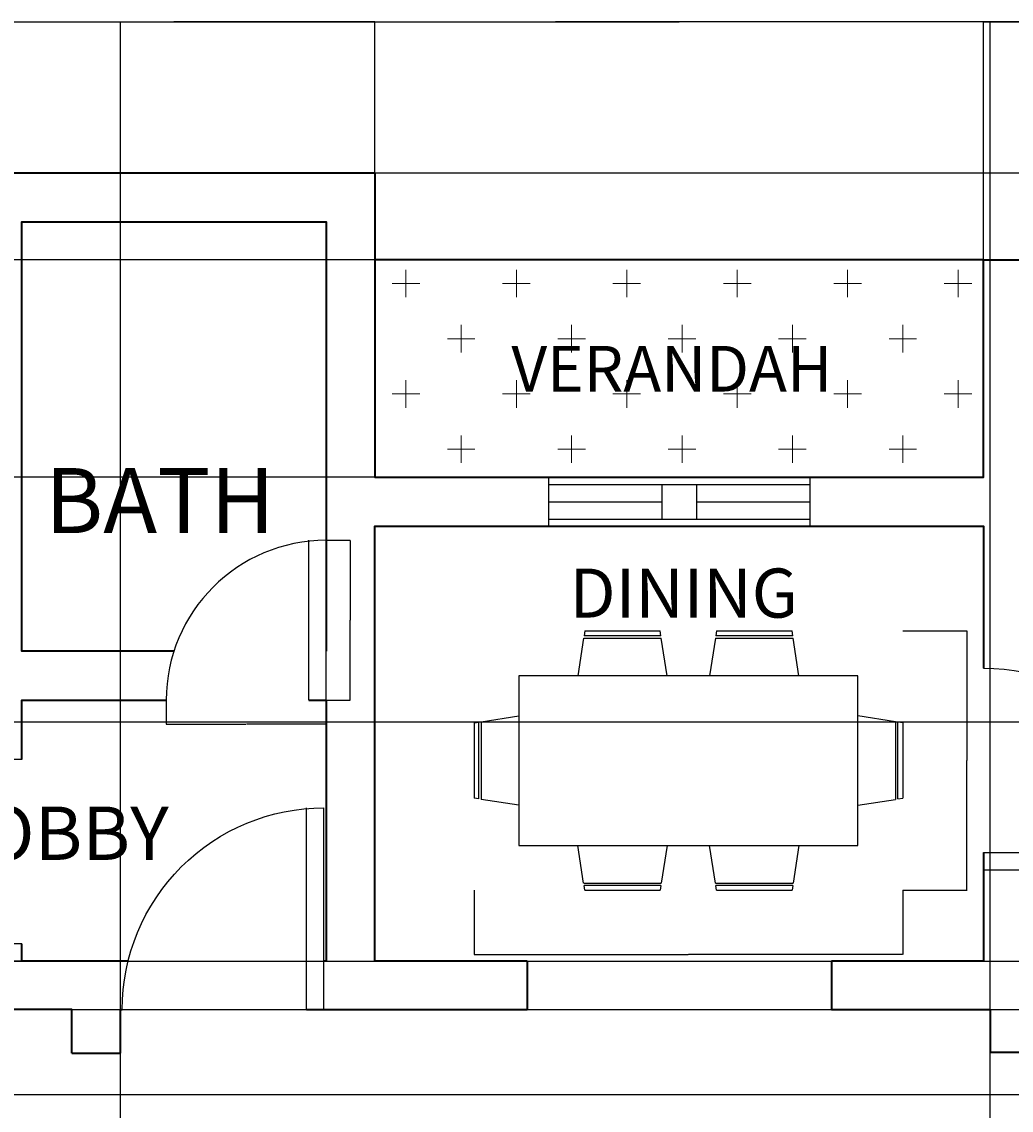
# Model space of a CAD drawing. Units: millimetres. Extents: x 19292 to 100733, y 12374 to 26974.
# Tile 17 of 24: x 26744 to 31296, y 18550 to 23556. Entities that reach past the tile are written whole.
import ezdxf

# ---------------------------------------------------------------- set-up
doc = ezdxf.new("R2010")
doc.units = ezdxf.units.MM
for name, color, linetype, lineweight in [('A-ANNO-DIMS', 2, 'Continuous', 18), ('A-AREA-IDEN', 3, 'Continuous', 25), ('A-DOOR', 4, 'Continuous', 25), ('A-FLOR-PATT', 252, 'Continuous', 13), ('A-FURN', 8, 'Continuous', 18), ('A-GLAZ', 3, 'Continuous', 25), ('A-WALL', 7, 'Continuous', 35)]:
    doc.layers.add(name, color=color, linetype=linetype, lineweight=lineweight)
doc.layers.add('FURNITURE', color=40, linetype='Continuous')
doc.layers.add('WINDOWS', color=50, linetype='Continuous')
doc.styles.get("Standard").update_dxf_attribs({"font": 'arial.ttf'})
doc.dimstyles.get("Standard").update_dxf_attribs({"dimtxt": 0.18, "dimasz": 0.18, "dimexe": 0.18, "dimexo": 0.0625, "dimgap": 0.09, "dimtad": 0, "dimtih": 1, "dimtoh": 1, "dimdec": 4, "dimzin": 0, "dimdsep": 46, "dimtxsty": 'Standard', "dimcen": 0.09, "dimadec": 0, "dimazin": 0, "dimtfac": 1, "dimtdec": 4, "dimtofl": 0, "dimtmove": 0, "dimatfit": 3, "dimfxl": 1, "dimtolj": 1, "dimtzin": 0, "dimarcsym": 0})

# ---------------------------------------------------------------- blocks, each defined once
blk = doc.blocks.new('WW')
at = {"layer": 'WINDOWS'}
for p, q in [((-5183.9, -4940.9), (-3983.9, -4940.9)), ((-4663.9, -4940.9), (-4663.9, -5100.9)), ((-4503.9, -4940.9), (-4503.9, -5100.9)), ((-4503.9, -4940.9), (-4503.9, -5100.9)), ((-5183.9, -5020.9), (-4663.9, -5020.9)), ((-4503.9, -5020.9), (-3983.9, -5020.9)), ((-5183.9, -5100.9), (-3983.9, -5100.9))]:
    blk.add_line(p, q, dxfattribs=at)
for points in [[(-5183.9, -5133.4), (-5183.9, -4908.4)], [(-3983.9, -4908.4), (-3983.9, -5133.4)]]:
    blk.add_lwpolyline(points, dxfattribs=at)
blk = doc.blocks.new('6X3DINING')
at = {"layer": 'FURNITURE'}
for p, q in [((13.7657, 44.00059), (12.5153, 35.99762)), ((13.7696, 44), (30.2392, 44)), ((14, 45.5), (13.8438, 44.50042)), ((30.1584, 44.5), (13.8466, 44.5)), ((14, 45.5), (30, 45.5)), ((30.1563, 44.49966), (30, 45.5)), ((31.4848, 35.99762), (30.2345, 43.99926)), ((41.7657, 44.00059), (40.5153, 35.99762)), ((41.7696, 44), (58.2392, 44)), ((42, 45.5), (41.8438, 44.50042)), ((58.1584, 44.5), (41.8466, 44.5)), ((42, 45.5), (58, 45.5)), ((58.1563, 44.49966), (58, 45.5)), ((59.4848, 35.99762), (58.2345, 43.99926)), ((72, 36), (0, 36)), ((0, 36), (0, 0)), ((72, 0), (72, 36)), ((-9.5, 26), (-8.5004, 26.15617)), ((-9.5, 26), (-9.5, 10)), ((-8.5, 9.84157), (-8.5, 26.15338)), ((-8.0006, 26.23428), (0.0024, 27.48474)), ((-8, 26.23041), (-8, 9.76085)), ((80.0006, 26.23428), (71.9976, 27.48474)), ((80, 26.23041), (80, 9.76085)), ((80.5, 9.84157), (80.5, 26.15338)), ((81.5, 26), (80.5005, 26.15617)), ((81.5, 26), (81.5, 10)), ((-8.4997, 9.84369), (-9.5, 10)), ((0.0024, 8.51524), (-7.9993, 9.7655)), ((71.9976, 8.51524), (79.9993, 9.7655)), ((80.4997, 9.84369), (81.5, 10)), ((0, 0), (72, 0)), ((13.7657, -8.0006), (12.5153, 0.00238)), ((31.4848, 0.00238), (30.2345, -7.99928)), ((41.7657, -8.0006), (40.5153, 0.00238)), ((59.4848, 0.00238), (58.2345, -7.99928)), ((13.7696, -8), (30.2392, -8)), ((14, -9.5), (13.8438, -8.50044)), ((30.1584, -8.5), (13.8466, -8.5)), ((30.1563, -8.49967), (30, -9.5)), ((41.7696, -8), (58.2392, -8)), ((42, -9.5), (41.8438, -8.50044)), ((58.1584, -8.5), (41.8466, -8.5)), ((58.1563, -8.49967), (58, -9.5)), ((14, -9.5), (30, -9.5)), ((42, -9.5), (58, -9.5))]:
    blk.add_line(p, q, dxfattribs=at)
blk = doc.blocks.new('DOOR-900')
for p, q in [((927.7, 80), (0, 80)), ((927.7, 0), (927.7, 80)), ((927.7, 0), (927.7, 80)), ((927.7, 0), (0, 0))]:
    blk.add_line(p, q)
blk.add_arc((927.7, 0), 927.7, 90, 180)
blk = doc.blocks.new('DOOR-750')
for p, q in [((655.3, 0), (655.3, 735.3)), ((735.3, 0), (735.3, 735.3)), ((735.3, 0), (655.3, 0)), ((735.3, 0), (655.3, 0))]:
    blk.add_line(p, q)
blk.add_arc((735.3, 0), 735.3, 90, 180)
blk = doc.blocks.new('DOOR-SWING-900')
blk.add_line((927.7, 927.7), (927.7, 0))
blk.add_arc((927.7, 927.7), 927.7, 180, 270)
blk = doc.blocks.new('*D30')
at = {"layer": 'A-ANNO-DIMS', "color": 0, "lineweight": -2, "transparency": 16777216}
for p, q in [((27408.9, 20435.7), (27408.9, 20325.3)), ((28144.1, 20435.7), (28144.1, 20325.3)), ((27409, 20325.4), (27775.2, 20325.4)), ((28144, 20325.4), (27777.7, 20325.4))]:
    blk.add_line(p, q, dxfattribs=at)
at = {"layer": 'A-ANNO-DIMS', "color": 0, "transparency": 16777216}
for points in [[(27409, 20325.5), (27409, 20325.4), (27408.9, 20325.4)], [(28144, 20325.5), (28144, 20325.4), (28144.1, 20325.4)]]:
    blk.add_solid(points, dxfattribs=at)
at = {"layer": 'Defpoints', "color": 0, "transparency": 16777216}
for p in [(27408.9, 20435.7), (28144.1, 20435.7), (28144.1, 20325.4)]:
    blk.add_point(p, dxfattribs=at)
at = {"layer": 'A-ANNO-DIMS', "color": 0, "transparency": 16777216, "insert": (27776.5, 20325.4), "char_height": 0.18, "attachment_point": 5}
blk.add_mtext('\\A1;DOOR 750 735 TYP.', dxfattribs=at)
blk = doc.blocks.new('*D31')
at = {"layer": 'A-ANNO-DIMS', "color": 0, "lineweight": -2, "transparency": 16777216}
for p, q in [((28144.2, 21171), (28254.6, 21171)), ((28254.4, 21170.8), (28254.4, 20803.5)), ((28254.4, 20435.9), (28254.4, 20803.2)), ((28144.2, 20435.7), (28254.6, 20435.7))]:
    blk.add_line(p, q, dxfattribs=at)
at = {"layer": 'A-ANNO-DIMS', "color": 0, "transparency": 16777216}
for points in [[(28254.4, 21170.8), (28254.5, 21170.8), (28254.4, 21171)], [(28254.4, 20435.9), (28254.5, 20435.9), (28254.4, 20435.7)]]:
    blk.add_solid(points, dxfattribs=at)
at = {"layer": 'Defpoints', "color": 0, "transparency": 16777216}
for p in [(28144.1, 21171), (28254.4, 21171), (28144.1, 20435.7)]:
    blk.add_point(p, dxfattribs=at)
at = {"layer": 'A-ANNO-DIMS', "color": 0, "transparency": 16777216, "insert": (28254.4, 20803.4), "char_height": 0.18, "attachment_point": 5}
blk.add_mtext('\\A1;735 TYP.', dxfattribs=at)
blk = doc.blocks.new('*D50')
at = {"layer": 'A-ANNO-DIMS', "color": 0, "lineweight": -2, "transparency": 16777216}
for p, q in [((28825.2, 19562.1), (28825.2, 19266.2)), ((30797.1, 19562.1), (30797.1, 19266.2)), ((28825.3, 19266.4), (29810, 19266.4)), ((30796.9, 19266.4), (29812.2, 19266.4))]:
    blk.add_line(p, q, dxfattribs=at)
at = {"layer": 'A-ANNO-DIMS', "color": 0, "transparency": 16777216}
for points in [[(28825.3, 19266.4), (28825.3, 19266.4), (28825.2, 19266.4)], [(30796.9, 19266.4), (30796.9, 19266.4), (30797.1, 19266.4)]]:
    blk.add_solid(points, dxfattribs=at)
at = {"layer": 'Defpoints', "color": 0, "transparency": 16777216}
for p in [(28825.2, 19562.2), (30797.1, 19562.2), (30797.1, 19266.4)]:
    blk.add_point(p, dxfattribs=at)
at = {"layer": 'A-ANNO-DIMS', "color": 0, "transparency": 16777216, "insert": (29811.1, 19266.4), "char_height": 0.18, "attachment_point": 5}
blk.add_mtext('\\A1;DINING SET 1972', dxfattribs=at)
blk = doc.blocks.new('*D51')
at = {"layer": 'A-ANNO-DIMS', "color": 0, "lineweight": -2, "transparency": 16777216}
for p, q in [((30797.1, 20754), (31093, 20754)), ((31092.8, 20753.8), (31092.8, 20158.2)), ((31092.8, 19562.3), (31092.8, 20157.9)), ((30797.1, 19562.2), (31093, 19562.2))]:
    blk.add_line(p, q, dxfattribs=at)
at = {"layer": 'A-ANNO-DIMS', "color": 0, "transparency": 16777216}
for points in [[(31092.8, 20753.8), (31092.9, 20753.8), (31092.8, 20754)], [(31092.8, 19562.3), (31092.9, 19562.3), (31092.8, 19562.2)]]:
    blk.add_solid(points, dxfattribs=at)
at = {"layer": 'Defpoints', "color": 0, "transparency": 16777216}
for p in [(30797.1, 20754), (31092.8, 20754), (30797.1, 19562.2)]:
    blk.add_point(p, dxfattribs=at)
at = {"layer": 'A-ANNO-DIMS', "color": 0, "transparency": 16777216, "insert": (31092.8, 20158.1), "char_height": 0.18, "attachment_point": 5}
blk.add_mtext('\\A1;1192', dxfattribs=at)
blk = doc.blocks.new('*D61')
at = {"layer": 'A-ANNO-DIMS', "color": 0, "lineweight": -2, "transparency": 16777216}
for p, q in [((26519.1, 22635.8), (26519.1, 23555.9)), ((26519.3, 23555.7), (27443.8, 23555.7)), ((28369, 23555.7), (27444.5, 23555.7)), ((28369.1, 22860.8), (28369.1, 23555.9))]:
    blk.add_line(p, q, dxfattribs=at)
at = {"layer": 'A-ANNO-DIMS', "color": 0, "transparency": 16777216}
for points in [[(26519.3, 23555.8), (26519.3, 23555.7), (26519.1, 23555.7)], [(28369, 23555.8), (28369, 23555.7), (28369.1, 23555.7)]]:
    blk.add_solid(points, dxfattribs=at)
at = {"layer": 'Defpoints', "color": 0, "transparency": 16777216}
for p in [(28369.1, 23555.7), (28369.1, 22860.7), (26519.1, 22635.7)]:
    blk.add_point(p, dxfattribs=at)
at = {"layer": 'A-ANNO-DIMS', "color": 0, "transparency": 16777216, "insert": (27444.1, 23555.7), "char_height": 0.18, "attachment_point": 5}
blk.add_mtext('\\A1;1850', dxfattribs=at)
blk = doc.blocks.new('*D62')
at = {"layer": 'A-ANNO-DIMS', "color": 0, "lineweight": -2, "transparency": 16777216}
for p, q in [((28369.132448, 22460.787437), (28369.132448, 23555.904937)), ((28369.312448, 23555.724937), (29768.772448, 23555.724937)), ((31168.952448, 23555.724937), (29769.492448, 23555.724937)), ((31169.132448, 22460.787437), (31169.132448, 23555.904937))]:
    blk.add_line(p, q, dxfattribs=at)
at = {"layer": 'A-ANNO-DIMS', "color": 0, "transparency": 16777216}
for points in [[(28369.312448, 23555.754937), (28369.312448, 23555.694937), (28369.132448, 23555.724937)], [(31168.952448, 23555.754937), (31168.952448, 23555.694937), (31169.132448, 23555.724937)]]:
    blk.add_solid(points, dxfattribs=at)
at = {"layer": 'Defpoints', "color": 0, "transparency": 16777216}
for p in [(31169.132448, 23555.724937), (28369.132448, 22460.724937), (31169.132448, 22460.724937)]:
    blk.add_point(p, dxfattribs=at)
at = {"layer": 'A-ANNO-DIMS', "color": 0, "transparency": 16777216, "insert": (29769.132448, 23555.724937), "char_height": 0.18, "attachment_point": 5}
blk.add_mtext('\\A1;2800', dxfattribs=at)
blk = doc.blocks.new('*D63')
at = {"layer": 'A-ANNO-DIMS', "color": 0, "lineweight": -2, "transparency": 16777216}
for p, q in [((31169.1, 22460.8), (31169.1, 23555.9)), ((31169.3, 23555.7), (31681.3, 23555.7)), ((32194, 23555.7), (31682, 23555.7)), ((32194.1, 22460.8), (32194.1, 23555.9))]:
    blk.add_line(p, q, dxfattribs=at)
at = {"layer": 'A-ANNO-DIMS', "color": 0, "transparency": 16777216}
for points in [[(31169.3, 23555.8), (31169.3, 23555.7), (31169.1, 23555.7)], [(32194, 23555.8), (32194, 23555.7), (32194.1, 23555.7)]]:
    blk.add_solid(points, dxfattribs=at)
at = {"layer": 'Defpoints', "color": 0, "transparency": 16777216}
for p in [(32194.1, 23555.7), (31169.1, 22460.7), (32194.1, 22460.7)]:
    blk.add_point(p, dxfattribs=at)
at = {"layer": 'A-ANNO-DIMS', "color": 0, "transparency": 16777216, "insert": (31681.6, 23555.7), "char_height": 0.18, "attachment_point": 5}
blk.add_mtext('\\A1;1025', dxfattribs=at)
blk = doc.blocks.new('*D68')
at = {"layer": 'A-ANNO-DIMS', "color": 0, "lineweight": -2, "transparency": 16777216}
for p, q in [((22919.2, 20335.7), (36879.3, 20335.7)), ((36879.2, 20335.5), (36879.2, 19785.9)), ((36879.2, 19235.9), (36879.2, 19785.5)), ((22919.2, 19235.7), (36879.3, 19235.7))]:
    blk.add_line(p, q, dxfattribs=at)
at = {"layer": 'A-ANNO-DIMS', "color": 0, "transparency": 16777216}
for points in [[(36879.1, 20335.5), (36879.2, 20335.5), (36879.2, 20335.7)], [(36879.1, 19235.9), (36879.2, 19235.9), (36879.2, 19235.7)]]:
    blk.add_solid(points, dxfattribs=at)
at = {"layer": 'Defpoints', "color": 0, "transparency": 16777216}
for p in [(22919.1, 20335.7), (22919.1, 19235.7), (36879.2, 19235.7)]:
    blk.add_point(p, dxfattribs=at)
at = {"layer": 'A-ANNO-DIMS', "color": 0, "transparency": 16777216, "insert": (36879.2, 19785.7), "char_height": 0.18, "attachment_point": 5}
blk.add_mtext('\\A1;1100', dxfattribs=at)
blk = doc.blocks.new('*D69')
at = {"layer": 'A-ANNO-DIMS', "color": 0, "lineweight": -2, "transparency": 16777216}
for p, q in [((23573.9, 19012.7), (36879.3, 19012.7)), ((36879.2, 19012.6), (36879.2, 18818)), ((36879.2, 18623), (36879.2, 18817.6)), ((23573.9, 18622.9), (36879.3, 18622.9))]:
    blk.add_line(p, q, dxfattribs=at)
at = {"layer": 'A-ANNO-DIMS', "color": 0, "transparency": 16777216}
for points in [[(36879.1, 19012.6), (36879.2, 19012.6), (36879.2, 19012.7)], [(36879.1, 18623), (36879.2, 18623), (36879.2, 18622.9)]]:
    blk.add_solid(points, dxfattribs=at)
at = {"layer": 'Defpoints', "color": 0, "transparency": 16777216}
for p in [(23573.8, 19012.7), (23573.8, 18622.9), (36879.2, 18622.9)]:
    blk.add_point(p, dxfattribs=at)
at = {"layer": 'A-ANNO-DIMS', "color": 0, "transparency": 16777216, "insert": (36879.2, 18817.8), "char_height": 0.18, "attachment_point": 5}
blk.add_mtext('\\A1;389.9', dxfattribs=at)
blk = doc.blocks.new('*D78')
at = {"layer": 'A-ANNO-DIMS', "color": 0, "lineweight": -2, "transparency": 16777216}
for p, q in [((28369.2, 22860.7), (36879.3, 22860.7)), ((36879.2, 22860.5), (36879.2, 22660.9)), ((36879.2, 22460.9), (36879.2, 22660.5)), ((36144.2, 22460.7), (36879.3, 22460.7))]:
    blk.add_line(p, q, dxfattribs=at)
at = {"layer": 'A-ANNO-DIMS', "color": 0, "transparency": 16777216}
for points in [[(36879.1, 22860.5), (36879.2, 22860.5), (36879.2, 22860.7)], [(36879.1, 22460.9), (36879.2, 22460.9), (36879.2, 22460.7)]]:
    blk.add_solid(points, dxfattribs=at)
at = {"layer": 'Defpoints', "color": 0, "transparency": 16777216}
for p in [(28369.1, 22860.7), (36879.2, 22860.7), (36144.1, 22460.7)]:
    blk.add_point(p, dxfattribs=at)
at = {"layer": 'A-ANNO-DIMS', "color": 0, "transparency": 16777216, "insert": (36879.2, 22660.7), "char_height": 0.18, "attachment_point": 5}
blk.add_mtext('\\A1;400', dxfattribs=at)
blk = doc.blocks.new('*D79')
at = {"layer": 'A-ANNO-DIMS', "color": 0, "lineweight": -2, "transparency": 16777216}
for p, q in [((22694.1, 22860.7), (22694.1, 12808.8)), ((36144.2, 15985.7), (36144.2, 12808.8)), ((22694.3, 12809), (29418.7, 12809)), ((36144, 12809), (29419.6, 12809))]:
    blk.add_line(p, q, dxfattribs=at)
at = {"layer": 'A-ANNO-DIMS', "color": 0, "transparency": 16777216}
for points in [[(22694.3, 12809), (22694.3, 12809), (22694.1, 12809)], [(36144, 12809), (36144, 12809), (36144.2, 12809)]]:
    blk.add_solid(points, dxfattribs=at)
at = {"layer": 'Defpoints', "color": 0, "transparency": 16777216}
for p in [(22694.1, 22860.7), (36144.2, 15985.7), (36144.2, 12809)]:
    blk.add_point(p, dxfattribs=at)
at = {"layer": 'A-ANNO-DIMS', "color": 0, "transparency": 16777216, "insert": (29419.2, 12809), "char_height": 0.18, "attachment_point": 5}
blk.add_mtext('\\A1;13450', dxfattribs=at)
blk = doc.blocks.new('*D82')
at = {"layer": 'A-ANNO-DIMS', "color": 0, "lineweight": -2, "transparency": 16777216}
for p, q in [((27198.8, 13562.8), (27198.8, 23555.9)), ((27199, 23555.7), (29296.4, 23555.7)), ((31394.6, 23555.7), (29297.2, 23555.7)), ((31394.8, 13544.1), (31394.8, 23555.9))]:
    blk.add_line(p, q, dxfattribs=at)
at = {"layer": 'A-ANNO-DIMS', "color": 0, "transparency": 16777216}
for points in [[(27199, 23555.8), (27199, 23555.7), (27198.8, 23555.7)], [(31394.6, 23555.8), (31394.6, 23555.7), (31394.8, 23555.7)]]:
    blk.add_solid(points, dxfattribs=at)
at = {"layer": 'Defpoints', "color": 0, "transparency": 16777216}
for p in [(31394.8, 23555.7), (27198.8, 13562.7), (31394.8, 13544)]:
    blk.add_point(p, dxfattribs=at)
at = {"layer": 'A-ANNO-DIMS', "color": 0, "transparency": 16777216, "insert": (29296.8, 23555.7), "char_height": 0.18, "attachment_point": 5}
blk.add_mtext('\\A1;4196', dxfattribs=at)
blk = doc.blocks.new('*D85')
at = {"layer": 'A-ANNO-DIMS', "color": 0, "lineweight": -2, "transparency": 16777216}
for p, q in [((31169.1, 22460.7), (21999, 22460.7)), ((21999.1, 22460.5), (21999.1, 21960.9)), ((21999.1, 21460.9), (21999.1, 21960.5)), ((31169.1, 21460.7), (21999, 21460.7))]:
    blk.add_line(p, q, dxfattribs=at)
at = {"layer": 'A-ANNO-DIMS', "color": 0, "transparency": 16777216}
for points in [[(21999.1, 22460.5), (21999.2, 22460.5), (21999.1, 22460.7)], [(21999.1, 21460.9), (21999.2, 21460.9), (21999.1, 21460.7)]]:
    blk.add_solid(points, dxfattribs=at)
at = {"layer": 'Defpoints', "color": 0, "transparency": 16777216}
for p in [(31169.1, 22460.7), (21999.1, 21460.7), (31169.1, 21460.7)]:
    blk.add_point(p, dxfattribs=at)
at = {"layer": 'A-ANNO-DIMS', "color": 0, "transparency": 16777216, "insert": (21999.1, 21960.7), "char_height": 0.18, "attachment_point": 5}
blk.add_mtext('\\A1;1000', dxfattribs=at)
blk = doc.blocks.new('*D86')
at = {"layer": 'A-ANNO-DIMS', "color": 0, "lineweight": -2, "transparency": 16777216}
for p, q in [((27198.8, 15132.8), (27198.8, 23555.9)), ((27199, 23555.7), (29198.5, 23555.7)), ((31198.6, 23555.7), (29199.2, 23555.7)), ((31198.8, 15132.8), (31198.8, 23555.9))]:
    blk.add_line(p, q, dxfattribs=at)
at = {"layer": 'A-ANNO-DIMS', "color": 0, "transparency": 16777216}
for points in [[(27199, 23555.8), (27199, 23555.7), (27198.8, 23555.7)], [(31198.6, 23555.8), (31198.6, 23555.7), (31198.8, 23555.7)]]:
    blk.add_solid(points, dxfattribs=at)
at = {"layer": 'Defpoints', "color": 0, "transparency": 16777216}
for p in [(31198.8, 23555.7), (27198.8, 15132.7), (31198.8, 15132.7)]:
    blk.add_point(p, dxfattribs=at)
at = {"layer": 'A-ANNO-DIMS', "color": 0, "transparency": 16777216, "insert": (29198.8, 23555.7), "char_height": 0.18, "attachment_point": 5}
blk.add_mtext('\\A1;4000', dxfattribs=at)

msp = doc.modelspace()

# ---------------------------------------------------------------- hatches: boundary and pattern name
at = {"layer": 'A-FLOR-PATT'}
h = msp.add_hatch(dxfattribs=at)
h.set_pattern_fill('CROSS', color=256, scale=40)
h.paths.add_polyline_path([(36144.169, 19010.725), (33719.169, 19010.725), (33719.169, 18850.725), (33719.169, 18003.026), (33719.169, 15985.725), (36144.169, 15985.725)])
h.paths.add_polyline_path([(36144.132, 22460.725), (34419.132, 22460.725), (34419.132, 22208.026, -0.34415073), (35121.831, 21308.026), (34419.132, 21308.026), (34419.132, 21260.725), (36144.132, 21260.725)])
h.paths.add_polyline_path([(34419.132, 22208.026), (34419.132, 21388.026), (35118.375, 21388.026, 0.32018294)], flags=17)
h.paths.add_polyline_path([(31169.132, 22460.725), (28369.132, 22460.725), (28369.132, 21460.725), (31169.132, 21460.725)])
h.paths.add_polyline_path([(34010.406, 17316.149), (36018.156, 17316.149), (36018.156, 17722.778), (34010.406, 17722.778)], flags=24)
h.paths.add_polyline_path([(34456.896, 21920.301), (35605.434, 21920.301), (35605.434, 22313.518), (34456.896, 22313.518)], flags=25)
h.paths.add_polyline_path([(29263.068, 21823.707), (30421.489, 21823.707), (30421.489, 22034.008), (29263.068, 22034.008)], flags=24)

# ---------------------------------------------------------------- linework, layer by layer
at = {"layer": 'A-DOOR'}
msp.add_line((31169.132, 19735.07), (32096.831, 19735.07), dxfattribs=at)
at = {"layer": 'A-WALL'}
for p, q in [((29069.132, 19235.725), (29069.132, 19012.748)), ((30469.132, 19235.725), (30469.132, 19012.748)), ((26973.815, 18812.748), (27198.815, 18812.748)), ((31394.132, 18815.368), (31198.815, 18815.368))]:
    msp.add_line(p, q, dxfattribs=at)
for points in [[(29548.571, 14906.403), (27198.815, 14906.403), (27198.815, 13562.748), (23348.815, 13562.748), (23348.815, 19010.725), (22694.132, 19010.725), (22694.132, 22860.725), (28369.132, 22860.725), (28369.132, 21460.725), (31169.132, 21460.725), (31169.132, 22460.725), (34419.132, 22460.725), (34419.132, 22208.026)], [(27444.132, 20660.725), (26744.132, 20660.725), (26744.132, 22635.725), (28144.132, 22635.725), (28144.132, 20660.725)], [(29069.132, 19235.725), (28369.132, 19235.725), (28369.132, 21235.725), (31169.132, 21235.725), (31169.132, 20582.769)], [(26744.132, 20163.424), (26744.132, 20435.725), (27408.86, 20435.725)], [(28064.132, 20435.725), (28144.132, 20435.725), (28144.132, 19235.725), (28133.974, 19235.725)], [(31169.132, 19735.07), (31169.132, 19235.725), (30469.132, 19235.725)], [(27233.47, 19235.725), (26744.132, 19235.725), (26744.132, 19315.725)], [(26973.815, 18812.748), (26973.815, 19012.748), (25728.446, 19012.748), (25728.446, 18622.462)], [(27198.815, 18812.748), (27198.815, 19012.748), (27206.275, 19012.748)], [(28053.974, 19012.748), (29069.132, 19012.748)], [(30469.132, 19012.748), (31198.815, 19012.748), (31198.815, 18815.368)]]:
    msp.add_lwpolyline(points, dxfattribs=at)
msp.add_lwpolyline([(28369.132, 21460.725), (31169.132, 21460.725), (31169.132, 22460.725), (28369.132, 22460.725)], close=True, dxfattribs=at)

# ---------------------------------------------------------------- block references
at = {"layer": 'A-DOOR'}
for name, p in [('DOOR-750', (27408.86, 20435.725)), ('DOOR-900', (25816.434, 19235.725))]:
    msp.add_blockref(name, p, dxfattribs=at)
at = {"layer": 'A-DOOR', "extrusion": (0, 0, -1), "zscale": -1}
for name, p, rotation in [('DOOR-SWING-900', (-32096.831, 20582.769), 269.9999999999995), ('DOOR-900', (-28133.973, 19940.446), 270.0000000000003)]:
    msp.add_blockref(name, p, dxfattribs=dict(at, rotation=rotation))
at = {"layer": 'A-FURN', "xscale": 21.6691686973019, "yscale": 21.6691686973019, "zscale": 21.6691686973019}
msp.add_blockref('6X3DINING', (29031.023, 19768.023), dxfattribs=at)
at = {"layer": 'A-GLAZ'}
msp.add_blockref('WW', (34353, 26369.102), dxfattribs=at)

# ---------------------------------------------------------------- texts
at = {"layer": 'A-AREA-IDEN'}
for s, height, p in [('VERANDAH', 209.9386, (28996.613, 21855.254)), ('BATH', 299.1707, (26850.797, 21204.251)), ('DINING', 225.7978, (29264.483, 20815.341)), ('LOBBY', 245.412, (26372.602, 19701.038))]:
    msp.add_text(s, height=height, dxfattribs=at).set_placement(p)

# ---------------------------------------------------------------- dimensions: what is measured, and where the dimension line sits
at = {"layer": 'A-ANNO-DIMS'}
for base, p1, p2, picture, middle in [((28369.132, 23555.725), (26519.132, 22635.725), (28369.132, 22860.725), '*D61', (27444.132, 23555.725)), ((31394.799, 23555.725), (27198.815, 13562.748), (31394.799, 13543.993), '*D82', (29296.807, 23555.725)), ((31198.815, 23555.725), (27198.815, 15132.748), (31198.815, 15132.748), '*D86', (29198.815, 23555.725)), ((31169.132, 23555.725), (28369.132, 22460.725), (31169.132, 22460.725), '*D62', (29769.132, 23555.725)), ((32194.132, 23555.725), (31169.132, 22460.725), (32194.132, 22460.725), '*D63', (31681.632, 23555.725)), ((36144.169, 12808.993), (22694.132, 22860.725), (36144.169, 15985.725), '*D79', (29419.151, 12808.993))]:
    dim = msp.add_linear_dim(base=base, p1=p1, p2=p2, dimstyle='Standard', override={"dimdec": 0, "dimlfac": 1, "dimrnd": 0, "dimzin": 0, "dimdsep": 46, "dimlunit": 2}, dxfattribs=at)
    dim.commit()
    dim.dimension.update_dxf_attribs({"geometry": picture, "text_midpoint": middle})
for base, p1, p2, override, picture, middle in [((36879.169, 22860.725), (36144.132, 22460.725), (28369.132, 22860.725), {"dimdec": 0, "dimlfac": 1, "dimrnd": 0, "dimzin": 0, "dimdsep": 46, "dimlunit": 2}, '*D78', (36879.169, 22660.725)), ((21999.132, 21460.725), (31169.132, 22460.725), (31169.132, 21460.725), {"dimdec": 0, "dimlfac": 1, "dimrnd": 0, "dimzin": 0, "dimdsep": 46, "dimlunit": 2}, '*D85', (21999.132, 21960.725)), ((31092.844, 20753.97), (30797.06, 19562.166), (30797.06, 20753.97), {"dimdec": 0, "dimrnd": 0, "dimzin": 0, "dimlunit": 2}, '*D51', (31092.844, 20158.068)), ((36879.169, 19235.725), (22919.132, 20335.725), (22919.132, 19235.725), {"dimdec": 0, "dimlfac": 1, "dimrnd": 0, "dimzin": 0, "dimdsep": 46, "dimlunit": 2}, '*D68', (36879.169, 19785.725)), ((36879.169, 18622.861), (23573.815, 19012.748), (23573.815, 18622.861), {"dimdec": 1, "dimlfac": 1, "dimrnd": 0, "dimzin": 0, "dimdsep": 46, "dimlunit": 2}, '*D69', (36879.169, 18817.804))]:
    dim = msp.add_linear_dim(base=base, p1=p1, p2=p2, angle=90, dimstyle='Standard', override=override, dxfattribs=at)
    dim.commit()
    dim.dimension.update_dxf_attribs({"geometry": picture, "text_midpoint": middle})
dim = msp.add_linear_dim(base=(28254.423, 21170.997), p1=(28144.132, 20435.725), p2=(28144.132, 21170.997), angle=90, text='<> TYP.', dimstyle='Standard', override={"dimdec": 0, "dimrnd": 0, "dimzin": 0, "dimlunit": 2}, dxfattribs=at)
dim.commit()
dim.dimension.update_dxf_attribs({"geometry": '*D31', "text_midpoint": (28254.423, 20803.361)})
for base, p1, p2, text, picture, middle in [((28144.132, 20325.434), (27408.86, 20435.725), (28144.132, 20435.725), 'DOOR 750 <> TYP.', '*D30', (27776.496, 20325.434)), ((30797.06, 19266.382), (28825.166, 19562.166), (30797.06, 19562.166), 'DINING SET <>', '*D50', (29811.113, 19266.382))]:
    dim = msp.add_linear_dim(base=base, p1=p1, p2=p2, text=text, dimstyle='Standard', override={"dimdec": 0, "dimrnd": 0, "dimzin": 0, "dimlunit": 2}, dxfattribs=at)
    dim.commit()
    dim.dimension.update_dxf_attribs({"geometry": picture, "text_midpoint": middle})

doc.saveas('drawing.dxf')
